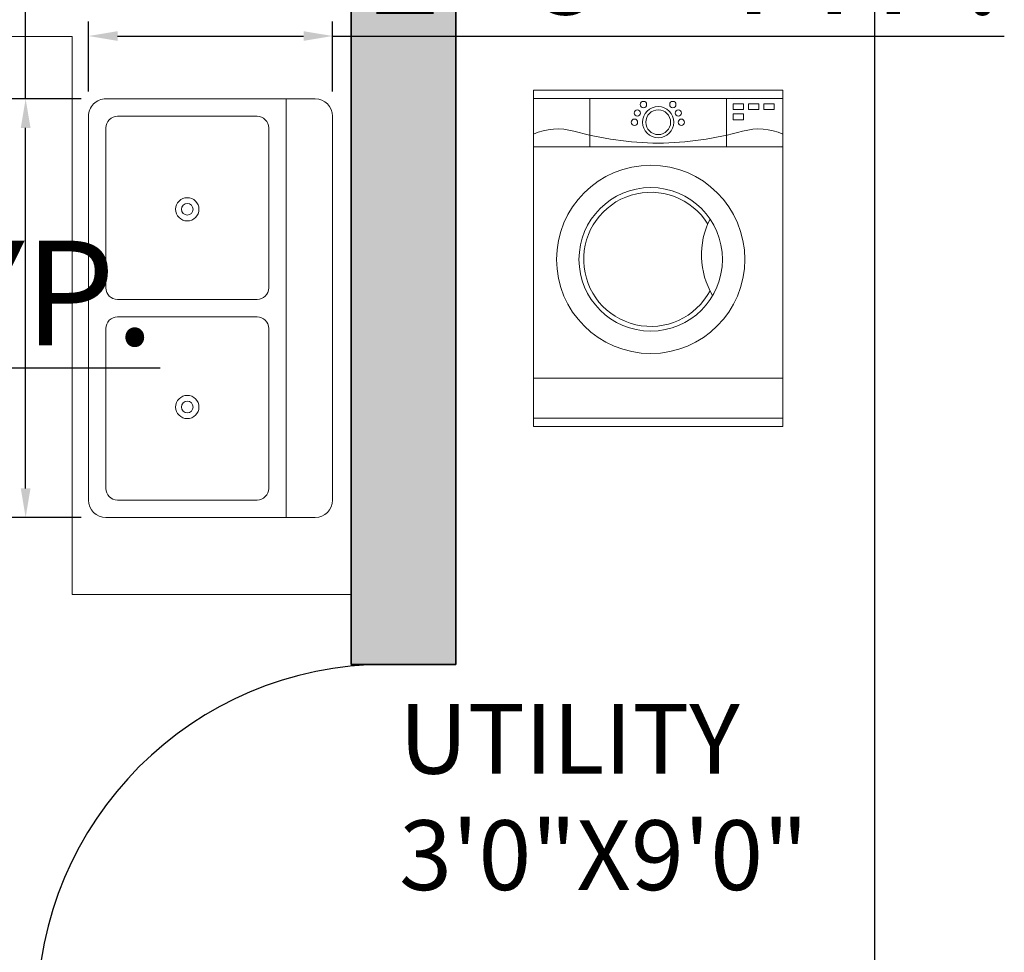
# Model space of a CAD drawing. Units: inches. Extents: x 2831 to 4250, y 1103 to 1797.
# Tile 11 of 15: x 3730 to 3814, y 1578 to 1658. Entities that reach past the tile are written whole.
import ezdxf

# ---------------------------------------------------------------- set-up
doc = ezdxf.new("R2010")
doc.units = ezdxf.units.IN
for name, color, linetype, lineweight in [('A-ANNO-DIMS', 2, 'Continuous', 18), ('A-AREA-IDEN', 7, 'Continuous', 18), ('A-DOOR', 4, 'Continuous', 25), ('A-EQPM', 8, 'Continuous', 18), ('A-FLOR-CASE', 9, 'Continuous', 18), ('A-WALL', 7, 'Continuous', 35), ('A-WALL-PATT', 252, 'Continuous', 13), ('C-PROP', 7, 'Continuous', 25), ('Сантехника', 9, 'Continuous', 18)]:
    doc.layers.add(name, color=color, linetype=linetype, lineweight=lineweight)
doc.styles.get("Standard").update_dxf_attribs({"font": 'arial.ttf'})
doc.dimstyles.new('ISO-25', dxfattribs={"dimtxt": 9, "dimasz": 2.5, "dimexe": 1.25, "dimexo": 0.625, "dimtad": 1, "dimdec": 1, "dimlunit": 3, "dimtxsty": 'Standard', "dimcen": 2.5, "dimadec": 0, "dimazin": 0, "dimtfac": 1, "dimtdec": 1, "dimtmove": 0, "dimatfit": 3, "dimfxl": 1, "dimarcsym": 0})

# ---------------------------------------------------------------- blocks, each defined once
blk = doc.blocks.new('*U4')
for p, q in [((0, 0), (0, -6)), ((30, 0), (30, -6))]:
    blk.add_line(p, q)
blk.add_lwpolyline([(0, 0), (0, 30), (1.75, 30), (1.75, 0)], close=True)
blk.add_arc((0, 0), 30, 0, 90)
blk = doc.blocks.new('Sink-double - 36 in top')
for p, q in [((-18, -4), (18, -4)), ((-0.75, -18.5), (-0.75, -6.5)), ((0.75, -6.5), (0.75, -18.5))]:
    blk.add_line(p, q)
for points in [[(-16.5, 0), (16.5, 0)], [(-18, -19.5), (-18, -1.5)], [(18, -1.5), (18, -19.5)], [(-15.5, -5.5), (-1.75, -5.5)], [(1.75, -5.5), (15.5, -5.5)], [(-16.5, -18.5), (-16.5, -6.5)], [(16.5, -6.5), (16.5, -18.5)], [(-1.75, -19.5), (-15.5, -19.5)], [(15.5, -19.5), (1.75, -19.5)], [(16.5, -21), (-16.5, -21)]]:
    blk.add_lwpolyline(points)
for centre, radius in [((-8.5, -12.5), 1), ((8.5, -12.5), 1), ((-8.5, -12.5), 0.5), ((8.5, -12.5), 0.5)]:
    blk.add_circle(centre, radius)
for centre, radius, start, end in [((-16.5, -1.5), 1.5, 90, 180), ((16.5, -1.5), 1.5, 0, 90), ((-15.5, -6.5), 1, 90, 180), ((-1.75, -6.5), 1, 0, 90), ((1.75, -6.5), 1, 90, 180), ((15.5, -6.5), 1, 0, 90), ((-15.5, -18.5), 1, 180, 270), ((-1.75, -18.5), 1, 270, 0), ((1.75, -18.5), 1, 180, 270), ((15.5, -18.5), 1, 270, 0), ((-16.5, -19.5), 1.5, 180, 270), ((16.5, -19.5), 1.5, 270, 0)]:
    blk.add_arc(centre, radius, start, end)
blk = doc.blocks.new('*D85')
at = {"layer": 'A-ANNO-DIMS', "color": 0, "lineweight": -2, "transparency": 16777216}
for p, q in [((3730.24, 1651.147), (3730.24, 1797.343)), ((3735.015, 1651.147), (3728.99, 1651.147)), ((3730.24, 1617.647), (3730.24, 1648.647)), ((3735.015, 1615.147), (3728.99, 1615.147))]:
    blk.add_line(p, q, dxfattribs=at)
at = {"layer": 'A-ANNO-DIMS', "color": 0, "transparency": 16777216}
for points in [[(3729.823, 1648.647), (3730.657, 1648.647), (3730.24, 1651.147)], [(3729.823, 1617.647), (3730.657, 1617.647), (3730.24, 1615.147)]]:
    blk.add_solid(points, dxfattribs=at)
at = {"layer": 'Defpoints', "color": 0, "transparency": 16777216}
for p in [(3730.24, 1651.147), (3735.64, 1651.147), (3735.64, 1615.147)]:
    blk.add_point(p, dxfattribs=at)
at = {"layer": 'A-ANNO-DIMS', "color": 0, "transparency": 16777216, "insert": (3724.955, 1725.495), "char_height": 9, "attachment_point": 5, "rotation": 90}
blk.add_mtext('DOUBLE SINK 3\'-0" TYP.', dxfattribs=at)
blk = doc.blocks.new('*D86')
at = {"layer": 'A-ANNO-DIMS', "color": 0, "lineweight": -2, "transparency": 16777216}
for p, q in [((3735.64, 1651.772), (3735.64, 1657.797)), ((3756.64, 1651.772), (3756.64, 1657.797)), ((3738.14, 1656.547), (3754.14, 1656.547)), ((3756.64, 1656.547), (3814.402, 1656.547))]:
    blk.add_line(p, q, dxfattribs=at)
at = {"layer": 'A-ANNO-DIMS', "color": 0, "transparency": 16777216}
for points in [[(3738.14, 1656.963), (3738.14, 1656.13), (3735.64, 1656.547)], [(3754.14, 1656.963), (3754.14, 1656.13), (3756.64, 1656.547)]]:
    blk.add_solid(points, dxfattribs=at)
at = {"layer": 'Defpoints', "color": 0, "transparency": 16777216}
for p in [(3756.64, 1656.547), (3735.64, 1651.147), (3756.64, 1651.147)]:
    blk.add_point(p, dxfattribs=at)
at = {"layer": 'A-ANNO-DIMS', "color": 0, "transparency": 16777216, "insert": (3786.771, 1661.767), "char_height": 9, "attachment_point": 5}
blk.add_mtext('1\'-9" TYP.', dxfattribs=at)
blk = doc.blocks.new('*D87')
at = {"layer": 'A-ANNO-DIMS', "color": 0, "lineweight": -2, "transparency": 16777216}
for p, q in [((3649.735, 1552.517), (3649.735, 1560.109)), ((3696.181, 1552.517), (3696.181, 1560.109)), ((3652.235, 1558.859), (3693.681, 1558.859)), ((3696.181, 1558.859), (3813.009, 1558.859))]:
    blk.add_line(p, q, dxfattribs=at)
at = {"layer": 'A-ANNO-DIMS', "color": 0, "transparency": 16777216}
for points in [[(3652.235, 1559.275), (3652.235, 1558.442), (3649.735, 1558.859)], [(3693.681, 1559.275), (3693.681, 1558.442), (3696.181, 1558.859)]]:
    blk.add_solid(points, dxfattribs=at)
at = {"layer": 'Defpoints', "color": 0, "transparency": 16777216}
for p in [(3696.181, 1558.859), (3649.735, 1551.892), (3696.181, 1551.892)]:
    blk.add_point(p, dxfattribs=at)
at = {"layer": 'A-ANNO-DIMS', "color": 0, "transparency": 16777216, "insert": (3755.845, 1564.143), "char_height": 9, "attachment_point": 5}
blk.add_mtext('HOB 3\'-10 1/2" TYP.', dxfattribs=at)
blk = doc.blocks.new('*D92')
at = {"layer": 'A-ANNO-DIMS', "color": 0, "lineweight": -2, "transparency": 16777216}
for p, q in [((3655.727, 1628.884), (3655.727, 1626.759)), ((3662.227, 1628.884), (3662.227, 1626.759)), ((3658.227, 1628.009), (3659.727, 1628.009)), ((3662.227, 1628.009), (3741.807, 1628.009))]:
    blk.add_line(p, q, dxfattribs=at)
at = {"layer": 'A-ANNO-DIMS', "color": 0, "transparency": 16777216}
for points in [[(3658.227, 1628.426), (3658.227, 1627.592), (3655.727, 1628.009)], [(3659.727, 1628.426), (3659.727, 1627.592), (3662.227, 1628.009)]]:
    blk.add_solid(points, dxfattribs=at)
at = {"layer": 'Defpoints', "color": 0, "transparency": 16777216}
for p in [(3655.727, 1629.509), (3662.227, 1629.509), (3662.227, 1628.009)]:
    blk.add_point(p, dxfattribs=at)
at = {"layer": 'A-ANNO-DIMS', "color": 0, "transparency": 16777216, "insert": (3703.267, 1633.287), "char_height": 9, "attachment_point": 5}
blk.add_mtext('0\'-6 1/2" TYP.', dxfattribs=at)

msp = doc.modelspace()

# ---------------------------------------------------------------- hatches: boundary and pattern name
at = {"layer": 'A-WALL-PATT'}
h = msp.add_hatch(color=256, dxfattribs=at)
h.dxf.hatch_style = 1
h.paths.add_polyline_path([(3479.227, 1418.513), (3488.227, 1418.513), (3488.227, 1426.809), (3488.227, 1460.513), (3588.227, 1460.513), (3588.227, 1466.513), (3488.227, 1466.513), (3488.227, 1470.513), (3479.227, 1470.513)])
h.paths.add_polyline_path([(3488.227, 1506.513), (3488.227, 1512.513), (3479.227, 1512.513), (3479.227, 1506.513)])
h.paths.add_polyline_path([(3488.227, 1370.513), (3479.227, 1370.513), (3479.227, 1319.513), (3521.227, 1319.513), (3521.227, 1328.513), (3488.227, 1328.513)])
h.paths.add_polyline_path([(3794.227, 1319.513), (3794.227, 1247.513), (3614.227, 1247.513), (3614.227, 1242.513), (3803.227, 1242.513), (3803.227, 1328.513), (3767.227, 1328.513), (3767.227, 1394.513), (3758.227, 1394.513), (3758.227, 1328.513), (3635.227, 1328.513), (3635.227, 1460.513), (3637.227, 1460.513), (3637.227, 1466.513), (3624.227, 1466.513), (3624.227, 1460.513), (3626.227, 1460.513), (3626.227, 1328.513), (3593.227, 1328.513), (3593.227, 1319.513)])
h.paths.add_polyline_path([(3758.227, 1460.513), (3758.227, 1442.513), (3767.227, 1442.513), (3767.227, 1460.513), (3783.227, 1460.513), (3783.227, 1492.513), (3774.227, 1492.513), (3774.227, 1466.513), (3761.32, 1466.513), (3726.227, 1466.513), (3726.227, 1468.513), (3720.227, 1468.513), (3720.227, 1466.513), (3673.227, 1466.513), (3673.227, 1460.513)])
h.paths.add_polyline_path([(3597.627, 1698.243), (3687.215, 1698.243), (3687.215, 1717.459), (3597.627, 1717.459)], flags=9)
h.paths.add_polyline_path([(3776.749, 1438.286), (3776.749, 1360.767), (3795.966, 1360.767), (3795.966, 1438.286)], flags=25)
h.paths.add_polyline_path([(3453.373, 1482.946), (3453.373, 1401.852), (3472.59, 1401.852), (3472.59, 1482.946)], flags=9)
h.paths.add_polyline_path([(3506.208, 1267.098), (3560.706, 1267.098), (3560.706, 1293.711), (3506.208, 1293.711)], flags=9)
h.paths.add_polyline_path([(3760.502, 1579.698), (3798.745, 1579.698), (3798.745, 1602.509), (3760.502, 1602.509)], flags=9)
h.paths.add_polyline_path([(3617.004, 1637.953), (3659.123, 1637.953), (3659.123, 1660.764), (3617.004, 1660.764)], flags=9)
h.paths.add_polyline_path([(3679.387, 1612.632), (3728.455, 1612.632), (3728.455, 1639.245), (3679.387, 1639.245)], flags=9)
h.paths.add_polyline_path([(3731.075, 1499.721), (3773.194, 1499.721), (3773.194, 1522.532), (3731.075, 1522.532)], flags=9)
h.paths.add_polyline_path([(3652.819, 1496.485), (3701.947, 1496.485), (3701.947, 1523.098), (3652.819, 1523.098)], flags=9)
h.paths.add_polyline_path([(3550.367, 1510.971), (3604.502, 1510.971), (3604.502, 1537.584), (3550.367, 1537.584)], flags=9)
h.paths.add_polyline_path([(3514.446, 1612.632), (3570.67, 1612.632), (3570.67, 1639.245), (3514.446, 1639.245)], flags=9)
h = msp.add_hatch(color=256, dxfattribs=at)
h.dxf.hatch_style = 1
h.paths.add_polyline_path([(3783.227, 1560.513), (3767.227, 1560.513), (3767.227, 1572.513), (3761.227, 1572.513), (3758.227, 1572.513), (3758.227, 1560.513), (3488.227, 1560.513), (3488.227, 1562.513), (3485.227, 1562.513), (3479.227, 1562.513), (3479.227, 1552.513), (3485.227, 1552.513), (3488.227, 1552.513), (3488.227, 1554.513), (3642.227, 1554.513), (3642.227, 1498.513), (3648.227, 1498.513), (3648.227, 1554.513), (3720.227, 1554.513), (3720.227, 1498.513), (3726.227, 1498.513), (3726.227, 1554.513), (3774.227, 1554.513), (3774.227, 1528.513), (3783.227, 1528.513)])
h.paths.add_polyline_path([(3767.227, 1689.513), (3728.227, 1689.513), (3728.227, 1680.513), (3758.227, 1680.513), (3758.227, 1602.513), (3767.227, 1602.513)])
h.paths.add_polyline_path([(3680.227, 1689.513), (3656.227, 1689.513), (3656.227, 1680.513), (3662.227, 1680.513), (3662.227, 1608.513), (3644.227, 1608.513), (3644.227, 1602.513), (3668.227, 1602.513), (3668.227, 1680.513), (3680.227, 1680.513)])
h.paths.add_polyline_path([(3620.227, 1689.513), (3584.227, 1689.513), (3584.227, 1680.513), (3608.227, 1680.513), (3608.227, 1602.513), (3614.227, 1602.513), (3614.227, 1608.513), (3614.227, 1638.513), (3614.227, 1680.513), (3620.227, 1680.513)])
h.paths.add_polyline_path([(3512.227, 1689.513), (3479.227, 1689.513), (3479.227, 1665.513), (3488.227, 1665.513), (3488.227, 1680.513), (3512.227, 1680.513)])
h.paths.add_polyline_path([(3488.227, 1617.513), (3479.227, 1617.513), (3479.227, 1602.513), (3485.227, 1602.513), (3488.227, 1602.513)])

# ---------------------------------------------------------------- linework, layer by layer
at = {"layer": 'A-EQPM'}
for p, q in [((3773.914, 1622.983), (3773.914, 1651.877)), ((3773.914, 1651.877), (3795.369, 1651.877)), ((3773.914, 1651.185), (3795.369, 1651.185)), ((3778.759, 1647.033), (3778.759, 1651.185)), ((3790.524, 1647.033), (3790.524, 1651.185)), ((3795.369, 1622.983), (3795.369, 1651.877)), ((3773.914, 1647.033), (3795.369, 1647.033)), ((3773.914, 1627.135), (3795.369, 1627.135)), ((3773.914, 1623.675), (3795.369, 1623.675)), ((3773.914, 1622.983), (3795.369, 1622.983))]:
    msp.add_line(p, q, dxfattribs=at)
for points in [[(3791.085, 1650.72), (3791.983, 1650.72), (3791.983, 1650.218), (3791.085, 1650.218)], [(3792.401, 1650.72), (3793.3, 1650.72), (3793.3, 1650.218), (3792.401, 1650.218)], [(3793.718, 1650.72), (3794.617, 1650.72), (3794.617, 1650.218), (3793.718, 1650.218)], [(3791.085, 1649.843), (3791.983, 1649.843), (3791.983, 1649.341), (3791.085, 1649.341)]]:
    msp.add_lwpolyline(points, close=True, dxfattribs=at)
for centre, radius in [((3783.369, 1650.657), 0.271), ((3784.641, 1649.134), 1.341), ((3785.897, 1650.657), 0.271), ((3782.845, 1649.926), 0.271), ((3784.641, 1649.134), 1.065), ((3786.377, 1649.926), 0.271), ((3782.596, 1649.134), 0.271), ((3786.629, 1649.134), 0.271), ((3783.994, 1637.343), 8.097), ((3783.994, 1637.343), 6.168)]:
    msp.add_circle(centre, radius, dxfattribs=at)
for centre, radius, start, end in [((3775.987, 1643.672), 4.886, 73.39316, 115.10502), ((3785.174, 1677.241), 29.919, 254.90635, 268.97939), ((3784.108, 1677.241), 29.919, 271.02061, 285.09365), ((3793.296, 1643.672), 4.886, 64.89498, 106.60684), ((3783.994, 1637.343), 5.768, 31.80671, 332.15064), ((3795.192, 1637.729), 6.833, 153.19, 210.76734)]:
    msp.add_arc(centre, radius, start, end, dxfattribs=at)
at = {"layer": 'A-FLOR-CASE'}
for p, q in [((3668.227, 1656.513), (3734.227, 1656.513)), ((3734.227, 1656.513), (3734.227, 1608.513)), ((3734.227, 1608.513), (3758.227, 1608.513))]:
    msp.add_line(p, q, dxfattribs=at)
at = {"layer": 'A-WALL'}
for p, q in [((3767.227, 1689.513), (3767.227, 1602.513)), ((3758.227, 1680.513), (3758.227, 1602.513)), ((3758.227, 1602.513), (3767.227, 1602.513))]:
    msp.add_line(p, q, dxfattribs=at)
at = {"layer": 'C-PROP'}
msp.add_lwpolyline([(3443.227, 1722.513), (3803.227, 1722.513), (3803.227, 1242.513), (3443.227, 1242.513)], close=True, dxfattribs=at)

# ---------------------------------------------------------------- block references
at = {"layer": 'A-DOOR', "rotation": 90}
msp.add_blockref('*U4', (3761.227, 1572.513), dxfattribs=at)
at = {"layer": 'Сантехника', "xscale": -1, "rotation": 270}
msp.add_blockref('Sink-double - 36 in top', (3756.64, 1633.147), dxfattribs=at)

# ---------------------------------------------------------------- texts
at = {"layer": 'A-AREA-IDEN', "insert": (3762.361, 1599.114), "char_height": 6, "attachment_point": 1}
msp.add_mtext_dynamic_manual_height_columns('{\\fTimes New Roman|b0|i0|c0|p18;UTILITY\\P3\'0"X9\'0"}', width=81.50747, gutter_width=12.5, heights=[0], dxfattribs=at)

# ---------------------------------------------------------------- dimensions: what is measured, and where the dimension line sits
at = {"layer": 'A-ANNO-DIMS'}
dim = msp.add_linear_dim(base=(3730.24, 1651.147), p1=(3735.64, 1615.147), p2=(3735.64, 1651.147), angle=90, text='DOUBLE SINK <> TYP.', dimstyle='ISO-25', override={"dimdec": 1, "dimlfac": 1, "dimrnd": 0, "dimzin": 1, "dimdsep": 46, "dimlunit": 4, "dimfrac": 2}, dxfattribs=at)
dim.commit()
dim.dimension.update_dxf_attribs({"geometry": '*D85', "text_midpoint": (3724.955, 1725.495)})
for base, p1, p2, text, picture, middle in [((3756.64, 1656.547), (3735.64, 1651.147), (3756.64, 1651.147), '<> TYP.', '*D86', (3786.771, 1661.767)), ((3662.227, 1628.009), (3655.727, 1629.509), (3662.227, 1629.509), '<> TYP.', '*D92', (3703.267, 1633.287)), ((3696.181, 1558.859), (3649.735, 1551.892), (3696.181, 1551.892), 'HOB <> TYP.', '*D87', (3755.845, 1564.143))]:
    dim = msp.add_linear_dim(base=base, p1=p1, p2=p2, text=text, dimstyle='ISO-25', override={"dimdec": 1, "dimlfac": 1, "dimrnd": 0, "dimzin": 1, "dimdsep": 46, "dimlunit": 4, "dimfrac": 2}, dxfattribs=at)
    dim.commit()
    dim.dimension.update_dxf_attribs({"geometry": picture, "text_midpoint": middle})

doc.saveas('drawing.dxf')
